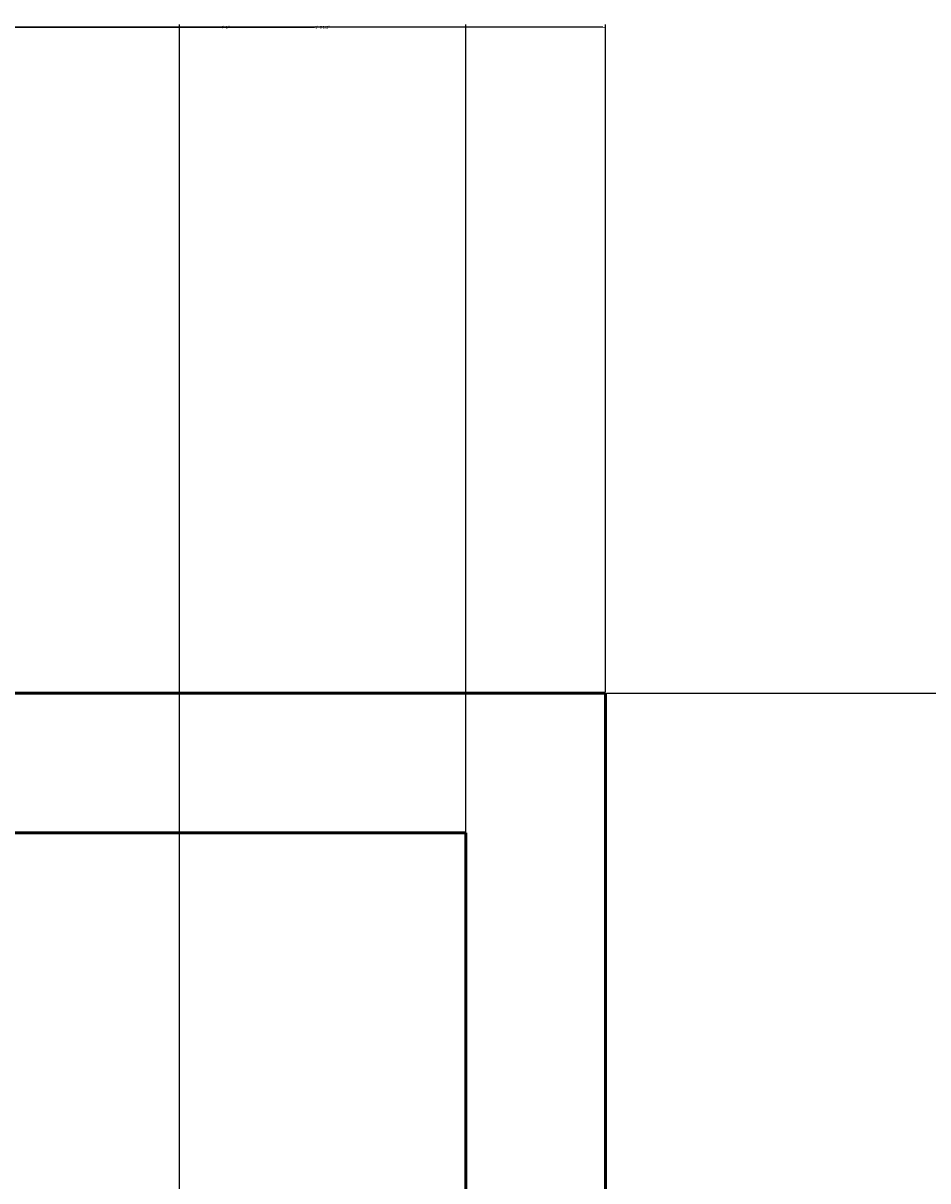
# Model space of a CAD drawing. Units: inches. Extents: x 37 to 824, y -700 to 234.
# Tile 76 of 77: x 391 to 449, y 160 to 234. Entities that reach past the tile are written whole.
import ezdxf

# ---------------------------------------------------------------- set-up
doc = ezdxf.new("R2010")
doc.units = ezdxf.units.IN
doc.header["$MEASUREMENT"] = 0
doc.layers.add('A-ANNO-DIMS', color=2, linetype='Continuous', lineweight=18)
doc.layers.add('A-WALL', color=2, linetype='Continuous', lineweight=50)
doc.styles.get("Standard").update_dxf_attribs({"font": 'arial.ttf'})
doc.dimstyles.get("Standard").update_dxf_attribs({"dimtxt": 0.18, "dimasz": 0.18, "dimexe": 0.18, "dimexo": 0.0625, "dimgap": 0.09, "dimtad": 0, "dimtih": 1, "dimtoh": 1, "dimdec": 1, "dimzin": 0, "dimdsep": 46, "dimlunit": 4, "dimtxsty": 'Standard', "dimcen": 0.09, "dimadec": 0, "dimazin": 0, "dimtfac": 1, "dimtdec": 1, "dimtofl": 0, "dimtmove": 0, "dimatfit": 3, "dimfxl": 1, "dimtolj": 1, "dimtzin": 0, "dimarcsym": 0})

# ---------------------------------------------------------------- blocks, each defined once
blk = doc.blocks.new('*D48')
at = {"layer": 'A-ANNO-DIMS', "color": 0, "lineweight": -2, "ltscale": 0.5, "transparency": 16777216}
for p, q in [((379.077, 191.153), (379.077, 234.17)), ((379.257, 233.99), (403.244, 233.99)), ((427.897, 233.99), (403.91, 233.99)), ((428.077, 191.153), (428.077, 234.17))]:
    blk.add_line(p, q, dxfattribs=at)
at = {"layer": 'A-ANNO-DIMS', "color": 0, "ltscale": 0.5, "transparency": 16777216}
for points in [[(379.257, 234.02), (379.257, 233.96), (379.077, 233.99)], [(427.897, 234.02), (427.897, 233.96), (428.077, 233.99)]]:
    blk.add_solid(points, dxfattribs=at)
at = {"layer": 'Defpoints', "color": 0, "ltscale": 0.5, "transparency": 16777216}
for p in [(428.077, 233.99), (379.077, 191.09), (428.077, 191.09)]:
    blk.add_point(p, dxfattribs=at)
at = {"layer": 'A-ANNO-DIMS', "color": 0, "ltscale": 0.5, "transparency": 16777216, "insert": (403.577, 233.99), "char_height": 0.18, "attachment_point": 5}
blk.add_mtext('\\A1;4\'-1"', dxfattribs=at)
blk = doc.blocks.new('*D63')
at = {"layer": 'A-ANNO-DIMS', "color": 0, "lineweight": -2, "ltscale": 0.5, "transparency": 16777216}
for p, q in [((161.077, 191.153), (161.077, 234.17)), ((161.257, 233.99), (294.176, 233.99)), ((427.897, 233.99), (294.978, 233.99)), ((428.077, 191.153), (428.077, 234.17))]:
    blk.add_line(p, q, dxfattribs=at)
at = {"layer": 'A-ANNO-DIMS', "color": 0, "ltscale": 0.5, "transparency": 16777216}
for points in [[(161.257, 234.02), (161.257, 233.96), (161.077, 233.99)], [(427.897, 234.02), (427.897, 233.96), (428.077, 233.99)]]:
    blk.add_solid(points, dxfattribs=at)
at = {"layer": 'Defpoints', "color": 0, "ltscale": 0.5, "transparency": 16777216}
for p in [(428.077, 233.99), (161.077, 191.09), (428.077, 191.09)]:
    blk.add_point(p, dxfattribs=at)
at = {"layer": 'A-ANNO-DIMS', "color": 0, "ltscale": 0.5, "transparency": 16777216, "insert": (294.577, 233.99), "char_height": 0.18, "attachment_point": 5}
blk.add_mtext('\\A1;22\'-3"', dxfattribs=at)
blk = doc.blocks.new('*D64')
at = {"layer": 'A-ANNO-DIMS', "color": 0, "lineweight": -2, "ltscale": 0.5, "transparency": 16777216}
for p, q in [((428.14, 191.09), (513.773, 191.09)), ((513.593, 190.91), (513.593, -87.228)), ((513.593, -365.73), (513.593, -87.591)), ((428.14, -365.91), (513.773, -365.91))]:
    blk.add_line(p, q, dxfattribs=at)
at = {"layer": 'A-ANNO-DIMS', "color": 0, "ltscale": 0.5, "transparency": 16777216}
for points in [[(513.563, 190.91), (513.623, 190.91), (513.593, 191.09)], [(513.563, -365.73), (513.623, -365.73), (513.593, -365.91)]]:
    blk.add_solid(points, dxfattribs=at)
at = {"layer": 'Defpoints', "color": 0, "ltscale": 0.5, "transparency": 16777216}
for p in [(428.077, 191.09), (428.077, -365.91), (513.593, -365.91)]:
    blk.add_point(p, dxfattribs=at)
at = {"layer": 'A-ANNO-DIMS', "color": 0, "ltscale": 0.5, "transparency": 16777216, "insert": (513.593, -87.41), "char_height": 0.18, "attachment_point": 5}
blk.add_mtext('\\A1;46\'-5"', dxfattribs=at)
blk = doc.blocks.new('*D74')
at = {"layer": 'A-ANNO-DIMS', "color": 0, "lineweight": -2, "ltscale": 0.5, "transparency": 16777216}
for p, q in [((371.077, 84.153), (371.077, 234.17)), ((371.257, 233.99), (385.3, 233.99)), ((400.425, 233.99), (386.381, 233.99)), ((400.605, 84.153), (400.605, 234.17))]:
    blk.add_line(p, q, dxfattribs=at)
at = {"layer": 'A-ANNO-DIMS', "color": 0, "ltscale": 0.5, "transparency": 16777216}
for points in [[(371.257, 234.02), (371.257, 233.96), (371.077, 233.99)], [(400.425, 234.02), (400.425, 233.96), (400.605, 233.99)]]:
    blk.add_solid(points, dxfattribs=at)
at = {"layer": 'Defpoints', "color": 0, "ltscale": 0.5, "transparency": 16777216}
for p in [(400.605, 233.99), (371.077, 84.09), (400.605, 84.09)]:
    blk.add_point(p, dxfattribs=at)
at = {"layer": 'A-ANNO-DIMS', "color": 0, "ltscale": 0.5, "transparency": 16777216, "insert": (385.841, 233.99), "char_height": 0.18, "attachment_point": 5}
blk.add_mtext('\\A1;2\'-5 1/2"', dxfattribs=at)
blk = doc.blocks.new('*D75')
at = {"layer": 'A-ANNO-DIMS', "color": 0, "lineweight": -2, "ltscale": 0.5, "transparency": 16777216}
for p, q in [((400.605, 84.153), (400.605, 234.17)), ((400.785, 233.99), (409.31, 233.99)), ((418.897, 233.99), (410.371, 233.99)), ((419.077, 84.153), (419.077, 234.17))]:
    blk.add_line(p, q, dxfattribs=at)
at = {"layer": 'A-ANNO-DIMS', "color": 0, "ltscale": 0.5, "transparency": 16777216}
for points in [[(400.785, 234.02), (400.785, 233.96), (400.605, 233.99)], [(418.897, 234.02), (418.897, 233.96), (419.077, 233.99)]]:
    blk.add_solid(points, dxfattribs=at)
at = {"layer": 'Defpoints', "color": 0, "ltscale": 0.5, "transparency": 16777216}
for p in [(419.077, 233.99), (400.605, 84.09), (419.077, 84.09)]:
    blk.add_point(p, dxfattribs=at)
at = {"layer": 'A-ANNO-DIMS', "color": 0, "ltscale": 0.5, "transparency": 16777216, "insert": (409.841, 233.99), "char_height": 0.18, "attachment_point": 5}
blk.add_mtext('\\A1;1\'-6 1/2"', dxfattribs=at)
blk = doc.blocks.new('*D83')
at = {"layer": 'A-ANNO-DIMS', "color": 0, "lineweight": -2, "ltscale": 0.5, "transparency": 16777216}
for p, q in [((358.132, -206.847), (358.132, 234.17)), ((358.312, 233.99), (388.275, 233.99)), ((418.897, 233.99), (388.934, 233.99)), ((419.077, -206.847), (419.077, 234.17))]:
    blk.add_line(p, q, dxfattribs=at)
at = {"layer": 'A-ANNO-DIMS', "color": 0, "ltscale": 0.5, "transparency": 16777216}
for points in [[(358.312, 234.02), (358.312, 233.96), (358.132, 233.99)], [(418.897, 234.02), (418.897, 233.96), (419.077, 233.99)]]:
    blk.add_solid(points, dxfattribs=at)
at = {"layer": 'Defpoints', "color": 0, "ltscale": 0.5, "transparency": 16777216}
for p in [(419.077, 233.99), (358.132, -206.91), (419.077, -206.91)]:
    blk.add_point(p, dxfattribs=at)
at = {"layer": 'A-ANNO-DIMS', "color": 0, "ltscale": 0.5, "transparency": 16777216, "insert": (388.605, 233.99), "char_height": 0.18, "attachment_point": 5}
blk.add_mtext('\\A1;5\'-1"', dxfattribs=at)

msp = doc.modelspace()

# ---------------------------------------------------------------- linework, layer by layer
at = {"layer": 'A-WALL'}
for p, q in [((299.077, 191.09), (428.077, 191.09)), ((428.077, 191.09), (428.077, 75.09)), ((299.077, 182.09), (419.077, 182.09)), ((419.077, 182.09), (419.077, 84.09))]:
    msp.add_line(p, q, dxfattribs=at)

# ---------------------------------------------------------------- dimensions: what is measured, and where the dimension line sits
at = {"layer": 'A-ANNO-DIMS', "ltscale": 0.5}
for base, p1, p2, picture, middle in [((400.605, 233.99), (371.077, 84.09), (400.605, 84.09), '*D74', (385.841, 233.99)), ((419.077, 233.99), (400.605, 84.09), (419.077, 84.09), '*D75', (409.841, 233.99)), ((428.077, 233.99), (161.077, 191.09), (428.077, 191.09), '*D63', (294.577, 233.99)), ((419.077, 233.99), (358.132, -206.91), (419.077, -206.91), '*D83', (388.605, 233.99)), ((428.077, 233.99), (379.077, 191.09), (428.077, 191.09), '*D48', (403.577, 233.99))]:
    dim = msp.add_linear_dim(base=base, p1=p1, p2=p2, dimstyle='Standard', override={"dimdec": 1, "dimlfac": 1, "dimrnd": 0, "dimzin": 1, "dimdsep": 46, "dimlunit": 4, "dimfrac": 2}, dxfattribs=at)
    dim.commit()
    dim.dimension.update_dxf_attribs({"geometry": picture, "text_midpoint": middle})
dim = msp.add_linear_dim(base=(513.593, -365.91), p1=(428.077, 191.09), p2=(428.077, -365.91), angle=90, dimstyle='Standard', override={"dimdec": 1, "dimlfac": 1, "dimrnd": 0, "dimzin": 1, "dimdsep": 46, "dimlunit": 4, "dimfrac": 2}, dxfattribs=at)
dim.commit()
dim.dimension.update_dxf_attribs({"geometry": '*D64', "text_midpoint": (513.593, -87.41)})

doc.saveas('drawing.dxf')
